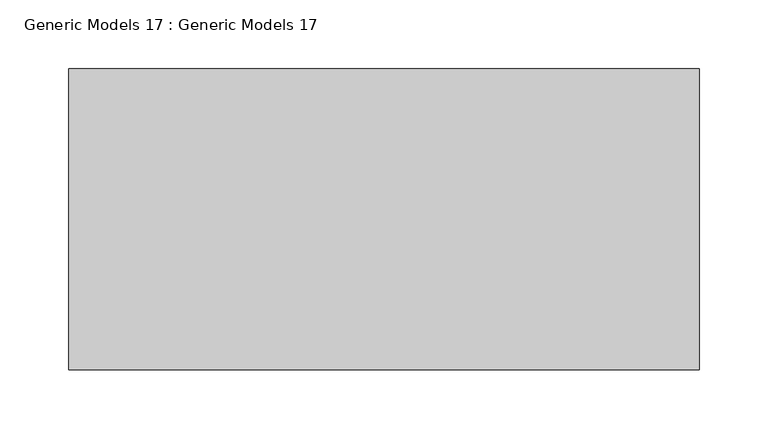
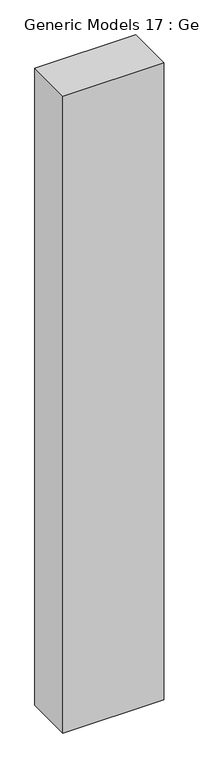
"""IFC4 building model written with IfcOpenShell, lengths in millimetres: proxy geometry, Generic Models 17 : Generic Models 17."""

from ifc_helpers import new_model, si_unit, origin, origin_with_axes, place, context, project, spatial, polyline, outline, extrude, source, transform, mapped, element, save


def generic_models_17_generic_models_17_b8611751(model_context):
    return source(origin(), model_context, "Body", "SweptSolid", [
        extrude(outline(polyline([(-9393.7642415, -5471.7273102), (-8936.5642415, -5471.7273102), (-8936.5642415, -5690.0708764), (-9393.7642415, -5690.0708764), (-9393.7642415, -5471.7273102)])), origin_with_axes(), (0.0, 0.0, 1.0), 3048.0),
    ])


if __name__ == "__main__":
    model = new_model("IFC4")
    model_context = context("Model", 3, world=origin())
    ifc_project = project(units=[si_unit("LENGTHUNIT", "METRE", prefix="MILLI")], contexts=[model_context])
    site = spatial("IfcSite", under=ifc_project)
    building = spatial("IfcBuilding", under=site)
    placement = place(None, origin())
    generic_models_17_generic_models_17_shape = generic_models_17_generic_models_17_b8611751(model_context)
    element("IfcBuildingElementProxy", 1, Name="Generic Models 17 : Generic Models 17", ObjectType="Generic Models 17 : Generic Models 17", at=placement, inside=building, context=model_context, shape_type="MappedRepresentation", body=[
        mapped(generic_models_17_generic_models_17_shape, transform((0.0, 0.0, 0.0), x_axis=(1.0, 0.0, 0.0), y_axis=(0.0, 1.0, 0.0), z_axis=(0.0, 0.0, 1.0))),
    ])
    save(model, "model.ifc")

# Revit data of these elements
# Element 1 (IfcBuildingElementProxy, "Generic Models 17 : Generic Models 17")
#   Materials on its faces: "exterior wall", "wall"
# Materials
#   "exterior wall": class "Generic", colour RGB 215 217 121, transparency 0, Cost = 0
#   "wall": class "Generic", colour RGB 127 127 127, transparency 0, Cost = 0
